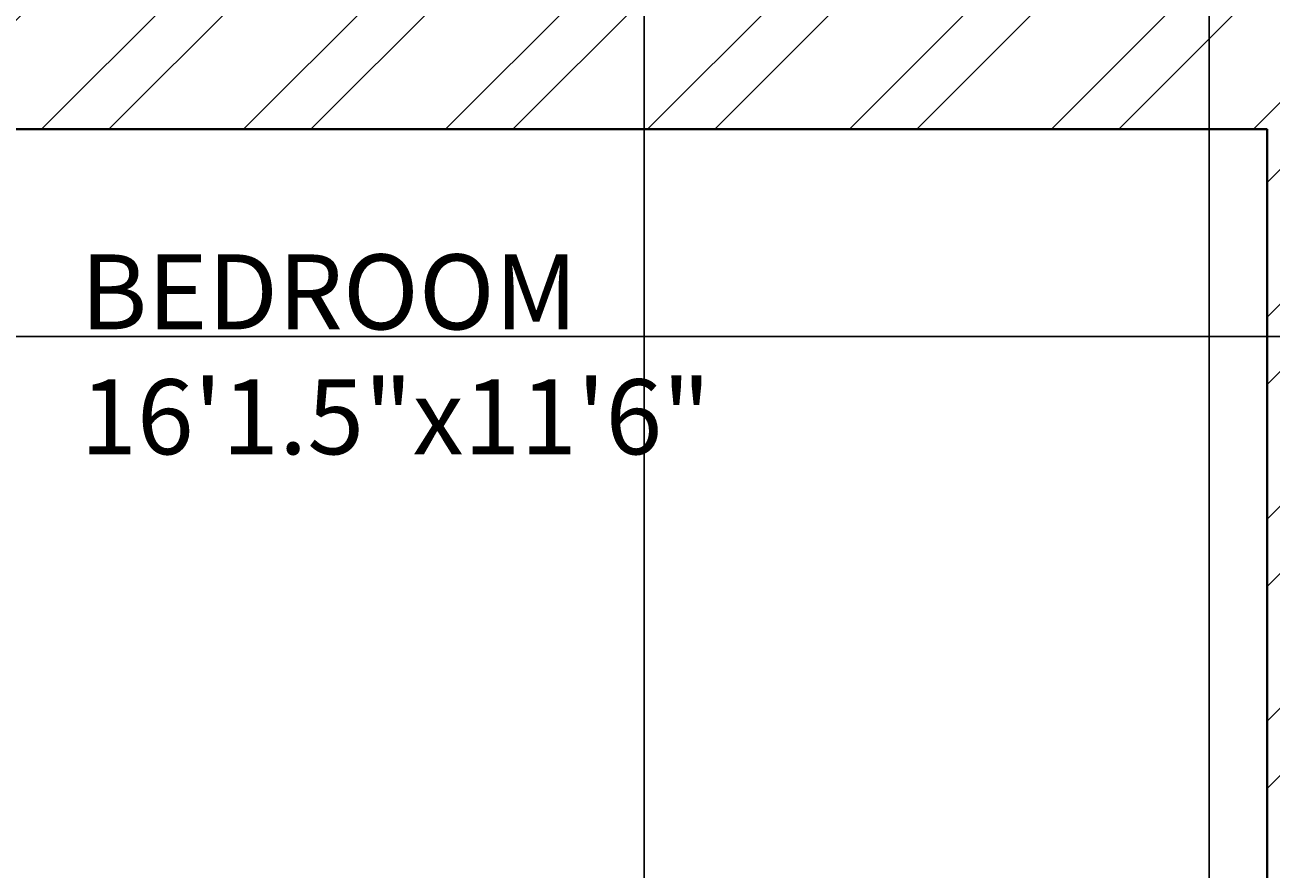
# Model space of a CAD drawing. Units: inches. Extents: x 1601 to 2297, y 1496 to 2631.
# Tile 13 of 57: x 1806 to 1889, y 1973 to 2029. Entities that reach past the tile are written whole.
import ezdxf

# ---------------------------------------------------------------- set-up
doc = ezdxf.new("R2010")
doc.units = ezdxf.units.IN
for name, color, linetype, lineweight in [('A-ANNO-DIMS', 2, 'Continuous', 18), ('A-AREA-IDEN', 7, 'Continuous', 18), ('A-WALL', 7, 'Continuous', 40), ('A-WALL-PATT', 215, 'Continuous', 13)]:
    doc.layers.add(name, color=color, linetype=linetype, lineweight=lineweight)
doc.styles.get("Standard").update_dxf_attribs({"font": 'arial.ttf'})
doc.dimstyles.get("Standard").update_dxf_attribs({"dimtxt": 0.18, "dimasz": 0.18, "dimexe": 0.18, "dimexo": 0.0625, "dimgap": 0.09, "dimtad": 0, "dimtih": 1, "dimtoh": 1, "dimdec": 4, "dimzin": 0, "dimdsep": 46, "dimtxsty": 'Standard', "dimcen": 0.09, "dimadec": 0, "dimazin": 0, "dimtfac": 1, "dimtdec": 4, "dimtofl": 0, "dimtmove": 0, "dimatfit": 3, "dimfxl": 1, "dimtolj": 1, "dimtzin": 0, "dimarcsym": 0})

# ---------------------------------------------------------------- blocks, each defined once
blk = doc.blocks.new('*D45')
at = {"layer": 'A-ANNO-DIMS', "color": 0, "lineweight": -2, "transparency": 16777216}
for p, q in [((1958.975, 2040.303), (1637.307, 2040.303)), ((1637.487, 2040.123), (1637.487, 2024.571)), ((1637.487, 2008.656), (1637.487, 2024.207)), ((1958.975, 2008.476), (1637.307, 2008.476))]:
    blk.add_line(p, q, dxfattribs=at)
at = {"layer": 'A-ANNO-DIMS', "color": 0, "transparency": 16777216}
for points in [[(1637.457, 2040.123), (1637.517, 2040.123), (1637.487, 2040.303)], [(1637.457, 2008.656), (1637.517, 2008.656), (1637.487, 2008.476)]]:
    blk.add_solid(points, dxfattribs=at)
at = {"layer": 'Defpoints', "color": 0, "transparency": 16777216}
for p in [(1637.487, 2040.303), (1959.037, 2040.303), (1959.037, 2008.476)]:
    blk.add_point(p, dxfattribs=at)
at = {"layer": 'A-ANNO-DIMS', "color": 0, "transparency": 16777216, "insert": (1637.487, 2024.389), "char_height": 0.18, "attachment_point": 5}
blk.add_mtext('\\A1;31.83', dxfattribs=at)
blk = doc.blocks.new('*D46')
at = {"layer": 'A-ANNO-DIMS', "color": 0, "lineweight": -2, "transparency": 16777216}
for p, q in [((1846.995, 2347.763), (1846.995, 1513.748)), ((1884.677, 2347.763), (1884.677, 1513.748)), ((1847.175, 1513.928), (1865.442, 1513.928)), ((1884.497, 1513.928), (1866.23, 1513.928))]:
    blk.add_line(p, q, dxfattribs=at)
at = {"layer": 'A-ANNO-DIMS', "color": 0, "transparency": 16777216}
for points in [[(1847.175, 1513.958), (1847.175, 1513.898), (1846.995, 1513.928)], [(1884.497, 1513.958), (1884.497, 1513.898), (1884.677, 1513.928)]]:
    blk.add_solid(points, dxfattribs=at)
at = {"layer": 'Defpoints', "color": 0, "transparency": 16777216}
for p in [(1846.995, 2347.825), (1884.677, 2347.825), (1884.677, 1513.928)]:
    blk.add_point(p, dxfattribs=at)
at = {"layer": 'A-ANNO-DIMS', "color": 0, "transparency": 16777216, "insert": (1865.836, 1513.928), "char_height": 0.18, "attachment_point": 5}
blk.add_mtext('\\A1;37.68', dxfattribs=at)

msp = doc.modelspace()

# ---------------------------------------------------------------- hatches: boundary and pattern name
at = {"layer": 'A-WALL-PATT'}
h = msp.add_hatch(dxfattribs=at)
h.set_pattern_fill('ANSI32', color=256)
h.paths.add_polyline_path([(1842.0336, 2528.0767), (1842.0336, 2532.3254), (1686.0373, 2532.3254), (1686.0373, 2492.9493), (1695.0373, 2492.9493), (1695.0373, 2523.3254), (1827.0373, 2523.3254), (1827.0373, 2416.8254), (1834.6225, 2416.8254), (1834.6225, 2419.0754), (1834.6225, 2421.3254), (1831.5373, 2421.3254), (1831.5373, 2523.3254), (1842.0336, 2523.3254)])
h.paths.add_polyline_path([(1695.0373, 2432.9493), (1686.0373, 2432.9493), (1686.0373, 2325.989), (1695.0373, 2325.989), (1695.0373, 2347.8254), (1827.0373, 2347.8254), (1827.0373, 2287.8254), (1823.2991, 2287.8254), (1823.2991, 2283.3254), (1847.9422, 2283.3254), (1847.9422, 2285.5754), (1847.9422, 2287.8254), (1831.5373, 2287.8254), (1831.5373, 2347.8254), (1846.9946, 2347.8254), (1846.9946, 2350.0754), (1846.9946, 2352.3254), (1695.0373, 2352.3254)])
h.paths.add_polyline_path([(1807.1169, 1573.5395), (2055.0405, 1573.5395), (2055.0405, 1610.6322), (1807.1169, 1610.6322)], flags=9)
h.paths.add_polyline_path([(1841.1631, 1712.7967), (1870.3957, 1712.7967), (1870.3957, 1731.454), (1841.1631, 1731.454)], flags=9)
h.paths.add_polyline_path([(2144.3862, 1772.185), (2191.0233, 1772.185), (2191.0233, 1790.8423), (2144.3862, 1790.8423)], flags=9)
h.paths.add_polyline_path([(2143.0128, 1827.3312), (2177.9958, 1827.3312), (2177.9958, 1845.9886), (2143.0128, 1845.9886)], flags=9)
h.paths.add_polyline_path([(2041.2439, 1833.5691), (2070.8516, 1833.5691), (2070.8516, 1852.2264), (2041.2439, 1852.2264)], flags=9)
h.paths.add_polyline_path([(2097.2791, 1947.0598), (2134.2061, 1947.0598), (2134.2061, 1965.7171), (2097.2791, 1965.7171)], flags=9)
h.paths.add_polyline_path([(2214.995, 1904.3124), (2214.995, 1942.2899), (2196.3376, 1942.2899), (2196.3376, 1904.3124)], flags=9)
h.paths.add_polyline_path([(2186.6284, 2043.8031), (2219.7935, 2043.8031), (2219.7935, 2062.4605), (2186.6284, 2062.4605)], flags=9)
h.paths.add_polyline_path([(2064.0877, 2031.616), (2097.4949, 2031.616), (2097.4949, 2050.2734), (2064.0877, 2050.2734)], flags=9)
h.paths.add_polyline_path([(1973.1349, 1986.0688), (2008.4009, 1986.0688), (2008.4009, 2004.7261), (1973.1349, 2004.7261)], flags=9)
h.paths.add_polyline_path([(1976.3676, 2106.9635), (2005.7469, 2106.9635), (2005.7469, 2125.6209), (1976.3676, 2125.6209)], flags=9)
h.paths.add_polyline_path([(1991.7852, 2180.4863), (2027.0513, 2180.4863), (2027.0513, 2199.1437), (1991.7852, 2199.1437)], flags=9)
h.paths.add_polyline_path([(2106.1801, 2187.9359), (2152.2101, 2187.9359), (2152.2101, 2206.5932), (2106.1801, 2206.5932)], flags=9)
h.paths.add_polyline_path([(2148.6686, 2262.2542), (2182.318, 2262.2542), (2182.318, 2280.9115), (2148.6686, 2280.9115)], flags=9)
h.paths.add_polyline_path([(2041.6327, 2252.8147), (2071.2405, 2252.8147), (2071.2405, 2271.4721), (2041.6327, 2271.4721)], flags=9)
h.paths.add_polyline_path([(2063.9734, 2375.4265), (2100.9004, 2375.4265), (2100.9004, 2394.0839), (2063.9734, 2394.0839)], flags=9)
h.paths.add_polyline_path([(2216.4955, 2330.9748), (2216.4955, 2370.2654), (2197.8381, 2370.2654), (2197.8381, 2330.9748)], flags=9)
h.paths.add_polyline_path([(2179.1416, 2485.8687), (2212.3067, 2485.8687), (2212.3067, 2504.5261), (2179.1416, 2504.5261)], flags=9)
h.paths.add_polyline_path([(2078.7442, 2471.1516), (2112.1514, 2471.1516), (2112.1514, 2489.809), (2078.7442, 2489.809)], flags=9)
h.paths.add_polyline_path([(1915.9631, 2329.4668), (1952.8902, 2329.4668), (1952.8902, 2348.1241), (1915.9631, 2348.1241)], flags=9)
h.paths.add_polyline_path([(1904.3189, 2499.6709), (1940.4512, 2499.6709), (1940.4512, 2518.3282), (1904.3189, 2518.3282)], flags=9)
h.paths.add_polyline_path([(1892.3665, 2100.4595), (1925.6374, 2100.4595), (1925.6374, 2119.1169), (1892.3665, 2119.1169)], flags=9)
h.paths.add_polyline_path([(1909.2984, 1805.9631), (1946.2254, 1805.9631), (1946.2254, 1824.6205), (1909.2984, 1824.6205)], flags=9)
h.paths.add_polyline_path([(1934.6056, 1658.616), (1970.738, 1658.616), (1970.738, 1677.2733), (1934.6056, 1677.2733)], flags=9)
h.paths.add_polyline_path([(1711.2052, 1789.8902), (1750.0456, 1789.8902), (1750.0456, 1808.5476), (1711.2052, 1808.5476)], flags=9)
h.paths.add_polyline_path([(1742.7874, 1854.6743), (1771.9449, 1854.6743), (1771.9449, 1873.3317), (1742.7874, 1873.3317)], flags=9)
h.paths.add_polyline_path([(1807.3592, 1997.7912), (1850.1116, 1997.7912), (1850.1116, 2016.4486), (1807.3592, 2016.4486)], flags=9)
h.paths.add_polyline_path([(1717.4579, 2237.7844), (1760.2103, 2237.7844), (1760.2103, 2256.4417), (1717.4579, 2256.4417)], flags=9)
h.paths.add_polyline_path([(1780.9285, 2324.0623), (1810.086, 2324.0623), (1810.086, 2342.7197), (1780.9285, 2342.7197)], flags=25)
h.paths.add_polyline_path([(1837.696, 2449.2024), (1866.9286, 2449.2024), (1866.9286, 2467.8598), (1837.696, 2467.8598)], flags=9)
h.paths.add_polyline_path([(1712.7752, 2484.9404), (1751.6156, 2484.9404), (1751.6156, 2503.5977), (1712.7752, 2503.5977)], flags=25)
h = msp.add_hatch(dxfattribs=at)
h.set_pattern_fill('ANSI32', color=256)
h.paths.add_polyline_path([(1973.9371, 2211.3254), (1893.0373, 2211.3254), (1893.0373, 2287.8254), (1884.6167, 2287.8254), (1884.6167, 2285.5754), (1884.6167, 2283.3254), (1888.5373, 2283.3254), (1888.5373, 2145.3254), (1695.0373, 2145.3254), (1695.0373, 2173.8724), (1690.5373, 2173.8724), (1686.0373, 2173.8724), (1686.0373, 2136.3254), (1722.5687, 2136.3254), (1722.5687, 2117.4352), (1731.5687, 2117.4352), (1731.5687, 2136.3254), (1893.0373, 2136.3254), (1893.0373, 2202.3254), (1959.0373, 2202.3254), (1959.0373, 2182.1303), (1968.0373, 2182.1303), (1968.0373, 2202.3254), (1973.9371, 2202.3254)])
h.paths.add_polyline_path([(2094.0373, 2274.6364), (2096.4294, 2274.6364), (2096.4294, 2276.8864), (2096.4294, 2279.1364), (2094.0373, 2279.1364), (2094.0373, 2290.8254), (2094.0373, 2295.3254), (2089.5373, 2295.3254), (2089.5373, 2230.8254), (2035.5373, 2230.8254), (2035.5373, 2299.8254), (2031.0373, 2299.8254), (2031.0373, 2211.3254), (2023.0065, 2211.3254), (2023.0065, 2202.3254), (2031.0373, 2202.3254), (2031.0373, 2140.8254), (1968.0373, 2140.8254), (1968.0373, 2145.9106), (1963.5373, 2145.9106), (1959.0373, 2145.9106), (1959.0373, 2116.839), (1963.5373, 2116.839), (1968.0373, 2116.839), (1968.0373, 2131.8254), (2031.0373, 2131.8254), (2031.0373, 2094.3254), (2031.0373, 2085.3254), (2031.0373, 2056.8254), (1968.0373, 2056.8254), (1968.0373, 2070.4947), (1963.5373, 2070.4947), (1959.0373, 2070.4947), (1959.0373, 2040.3029), (1968.0373, 2040.3029), (1968.0373, 2047.8254), (2031.0373, 2047.8254), (2031.0373, 1983.3254), (2031.0373, 1978.8254), (2021.1979, 1978.8254), (2021.1979, 1974.3254), (2031.0373, 1974.3254), (2031.0373, 1954.3528), (2035.5373, 1954.3528), (2035.5373, 1974.3254), (2035.5373, 1981.8254), (2055.5513, 1981.8254), (2055.5513, 1986.3254), (2035.5373, 1986.3254), (2035.5373, 2047.8254), (2040.0373, 2047.8254), (2040.0373, 2085.3254), (2040.0373, 2094.3254), (2040.0373, 2140.8254), (2035.5373, 2140.8254), (2035.5373, 2226.3254), (2089.5373, 2226.3254), (2094.0373, 2226.3254)])
h.paths.add_polyline_path([(2226.0373, 2230.8254), (2134.5373, 2230.8254), (2134.5373, 2233.5437), (2130.0373, 2233.5437), (2130.0373, 2226.3254), (2134.5373, 2226.3254), (2226.0373, 2226.3254)])
h.paths.add_polyline_path([(1807.1169, 1573.5395), (2055.0405, 1573.5395), (2055.0405, 1610.6322), (1807.1169, 1610.6322)], flags=9)
h.paths.add_polyline_path([(1841.1631, 1712.7967), (1870.3957, 1712.7967), (1870.3957, 1731.454), (1841.1631, 1731.454)], flags=9)
h.paths.add_polyline_path([(2144.3862, 1772.185), (2191.0233, 1772.185), (2191.0233, 1790.8423), (2144.3862, 1790.8423)], flags=9)
h.paths.add_polyline_path([(2143.0128, 1827.3312), (2177.9958, 1827.3312), (2177.9958, 1845.9886), (2143.0128, 1845.9886)], flags=9)
h.paths.add_polyline_path([(2041.2439, 1833.5691), (2070.8516, 1833.5691), (2070.8516, 1852.2264), (2041.2439, 1852.2264)], flags=9)
h.paths.add_polyline_path([(2097.2791, 1947.0598), (2134.2061, 1947.0598), (2134.2061, 1965.7171), (2097.2791, 1965.7171)], flags=9)
h.paths.add_polyline_path([(2214.995, 1904.3124), (2214.995, 1942.2899), (2196.3376, 1942.2899), (2196.3376, 1904.3124)], flags=9)
h.paths.add_polyline_path([(2186.6284, 2043.8031), (2219.7935, 2043.8031), (2219.7935, 2062.4605), (2186.6284, 2062.4605)], flags=9)
h.paths.add_polyline_path([(2064.0877, 2031.616), (2097.4949, 2031.616), (2097.4949, 2050.2734), (2064.0877, 2050.2734)], flags=9)
h.paths.add_polyline_path([(1973.1349, 1986.0688), (2008.4009, 1986.0688), (2008.4009, 2004.7261), (1973.1349, 2004.7261)], flags=25)
h.paths.add_polyline_path([(1976.3676, 2106.9635), (2005.7469, 2106.9635), (2005.7469, 2125.6209), (1976.3676, 2125.6209)], flags=25)
h.paths.add_polyline_path([(1991.7852, 2180.4863), (2027.0513, 2180.4863), (2027.0513, 2199.1437), (1991.7852, 2199.1437)], flags=25)
h.paths.add_polyline_path([(2106.1801, 2187.9359), (2152.2101, 2187.9359), (2152.2101, 2206.5932), (2106.1801, 2206.5932)], flags=9)
h.paths.add_polyline_path([(2148.6686, 2262.2542), (2182.318, 2262.2542), (2182.318, 2280.9115), (2148.6686, 2280.9115)], flags=9)
h.paths.add_polyline_path([(2041.6327, 2252.8147), (2071.2405, 2252.8147), (2071.2405, 2271.4721), (2041.6327, 2271.4721)], flags=25)
h.paths.add_polyline_path([(2063.9734, 2375.4265), (2100.9004, 2375.4265), (2100.9004, 2394.0839), (2063.9734, 2394.0839)], flags=9)
h.paths.add_polyline_path([(2216.4955, 2330.9748), (2216.4955, 2370.2654), (2197.8381, 2370.2654), (2197.8381, 2330.9748)], flags=9)
h.paths.add_polyline_path([(2179.1416, 2485.8687), (2212.3067, 2485.8687), (2212.3067, 2504.5261), (2179.1416, 2504.5261)], flags=9)
h.paths.add_polyline_path([(2078.7442, 2471.1516), (2112.1514, 2471.1516), (2112.1514, 2489.809), (2078.7442, 2489.809)], flags=9)
h.paths.add_polyline_path([(1915.9631, 2329.4668), (1952.8902, 2329.4668), (1952.8902, 2348.1241), (1915.9631, 2348.1241)], flags=9)
h.paths.add_polyline_path([(1904.3189, 2499.6709), (1940.4512, 2499.6709), (1940.4512, 2518.3282), (1904.3189, 2518.3282)], flags=9)
h.paths.add_polyline_path([(1892.3665, 2100.4595), (1925.6374, 2100.4595), (1925.6374, 2119.1169), (1892.3665, 2119.1169)], flags=9)
h.paths.add_polyline_path([(1909.2984, 1805.9631), (1946.2254, 1805.9631), (1946.2254, 1824.6205), (1909.2984, 1824.6205)], flags=9)
h.paths.add_polyline_path([(1934.6056, 1658.616), (1970.738, 1658.616), (1970.738, 1677.2733), (1934.6056, 1677.2733)], flags=9)
h.paths.add_polyline_path([(1711.2052, 1789.8902), (1750.0456, 1789.8902), (1750.0456, 1808.5476), (1711.2052, 1808.5476)], flags=9)
h.paths.add_polyline_path([(1742.7874, 1854.6743), (1771.9449, 1854.6743), (1771.9449, 1873.3317), (1742.7874, 1873.3317)], flags=9)
h.paths.add_polyline_path([(1807.3592, 1997.7912), (1850.1116, 1997.7912), (1850.1116, 2016.4486), (1807.3592, 2016.4486)], flags=9)
h.paths.add_polyline_path([(1717.4579, 2237.7844), (1760.2103, 2237.7844), (1760.2103, 2256.4417), (1717.4579, 2256.4417)], flags=25)
h.paths.add_polyline_path([(1780.9285, 2324.0623), (1810.086, 2324.0623), (1810.086, 2342.7197), (1780.9285, 2342.7197)], flags=9)
h.paths.add_polyline_path([(1837.696, 2449.2024), (1866.9286, 2449.2024), (1866.9286, 2467.8598), (1837.696, 2467.8598)], flags=9)
h.paths.add_polyline_path([(1712.7752, 2484.9404), (1751.6156, 2484.9404), (1751.6156, 2503.5977), (1712.7752, 2503.5977)], flags=9)
h = msp.add_hatch(dxfattribs=at)
h.set_pattern_fill('ANSI32', color=256)
h.paths.add_polyline_path([(2230.5373, 1861.8254), (2182.5373, 1861.8254), (2182.5373, 1885.3637), (2178.0373, 1885.3637), (2178.0373, 1861.8254), (2166.0373, 1861.8254), (2134.5373, 1861.8254), (2130.0373, 1861.8254), (2130.0373, 1841.4682), (2126.8833, 1841.4682), (2126.8833, 1836.9682), (2130.0373, 1836.9682), (2130.0373, 1822.7302), (2134.5373, 1822.7302), (2134.5373, 1857.3254), (2166.0373, 1857.3254), (2226.0373, 1857.3254), (2226.0373, 1846.1155), (2230.5373, 1846.1155)])
h.paths.add_polyline_path([(2226.0373, 1797.3254), (2134.5373, 1797.3254), (2134.5373, 1800.6636), (2132.2873, 1800.6636), (2130.0373, 1800.6636), (2130.0373, 1797.3254), (2130.0373, 1792.8254), (2167.7264, 1792.8254), (2226.0373, 1792.8254)])
h.paths.add_polyline_path([(2230.5373, 1822.1155), (2226.0373, 1822.1155), (2226.0373, 1760.8563), (2230.5373, 1760.8563)])
h.paths.add_polyline_path([(2230.5373, 1700.8563), (2226.0373, 1700.8563), (2226.0373, 1644.3254), (2140.2517, 1644.3254), (2140.2517, 1635.3254), (2230.5373, 1635.3254)])
h.paths.add_polyline_path([(2080.2517, 1639.8254), (2080.2517, 1644.3254), (2035.5373, 1644.3254), (2035.5373, 1792.8254), (2094.0373, 1792.8254), (2094.0373, 1797.3254), (2094.0373, 1836.9682), (2097.1057, 1836.9682), (2097.1057, 1839.2182), (2097.1057, 1841.4682), (2094.0373, 1841.4682), (2094.0373, 1862.2276), (2089.5373, 1862.2276), (2089.5373, 1797.3254), (2035.5373, 1797.3254), (2035.5373, 1857.3254), (2035.5373, 1885.0916), (2031.0373, 1885.0916), (2031.0373, 1710.3254), (2012.329, 1710.3254), (2012.329, 1701.3254), (2031.0373, 1701.3254), (2031.0373, 1644.3254), (2031.0373, 1635.3254), (2080.2517, 1635.3254)])
h.paths.add_polyline_path([(1836.0373, 1653.2033), (1842.6171, 1653.2033), (1842.6171, 1657.7033), (1842.6171, 1662.2033), (1831.5373, 1662.2033), (1831.5373, 1764.2033), (1835.3881, 1764.2033), (1835.3881, 1766.4533), (1835.3881, 1768.7033), (1831.5373, 1768.7033), (1827.0373, 1768.7033), (1827.0373, 1662.2033), (1827.0373, 1635.3254), (1836.0373, 1635.3254)])
h.paths.add_polyline_path([(1893.0373, 1701.3254), (1907.193, 1701.3254), (1907.193, 1705.8254), (1907.193, 1710.3254), (1893.0373, 1710.3254), (1893.0373, 1819.8254), (1882.6444, 1819.8254), (1882.6444, 1817.5754), (1882.6444, 1815.3254), (1888.5373, 1815.3254), (1888.5373, 1662.2033), (1884.0373, 1662.2033), (1866.6171, 1662.2033), (1866.6171, 1653.2033), (1882.391, 1653.2033), (1884.0373, 1653.2033), (1884.0373, 1635.3254), (1893.0373, 1635.3254)])
h.paths.add_polyline_path([(1739.3335, 1639.8254), (1739.3335, 1644.3254), (1695.0373, 1644.3254), (1695.0373, 1702.0135), (1690.5373, 1702.0135), (1686.0373, 1702.0135), (1686.0373, 1635.3254), (1739.3335, 1635.3254)])
h.paths.add_polyline_path([(1827.0373, 1644.3254), (1799.3335, 1644.3254), (1799.3335, 1635.3254), (1827.0373, 1635.3254)])
h.paths.add_polyline_path([(1695.0373, 1815.3254), (1849.2759, 1815.3254), (1849.2759, 1819.8254), (1807.5373, 1819.8254), (1807.5373, 1879.8254), (1851.1533, 1879.8254), (1851.1533, 1882.0754), (1851.1533, 1884.3254), (1799.3405, 1884.3254), (1799.3405, 1882.0754), (1799.3405, 1879.8254), (1803.0373, 1879.8254), (1803.0373, 1819.8254), (1695.0373, 1819.8254), (1695.0373, 1835.0458), (1690.5373, 1835.0458), (1686.0373, 1835.0458), (1686.0373, 1766.1753), (1695.0373, 1766.1753)])
h.paths.add_polyline_path([(1775.8157, 1884.3254), (1695.0373, 1884.3254), (1695.0373, 1912.9526), (1690.5373, 1912.9526), (1686.0373, 1912.9526), (1686.0373, 1859.0458), (1695.0373, 1859.0458), (1695.0373, 1879.8254), (1775.8157, 1879.8254)])
h.paths.add_polyline_path([(1893.0373, 2031.3254), (1731.5687, 2031.3254), (1731.5687, 2057.4352), (1722.5687, 2057.4352), (1722.5687, 2031.3254), (1686.0373, 2031.3254), (1686.0373, 1972.9526), (1695.0373, 1972.9526), (1695.0373, 2022.3254), (1888.5373, 2022.3254), (1888.5373, 1884.3254), (1883.4996, 1884.3254), (1883.4996, 1879.8254), (1893.0373, 1879.8254), (1893.0373, 1974.3254), (1976.6199, 1974.3254), (1976.6199, 1978.8254), (1968.0373, 1978.8254), (1968.0373, 1983.3254), (1968.0373, 2008.4756), (1963.5373, 2008.4756), (1959.0373, 2008.4756), (1959.0373, 1983.3254), (1893.0373, 1983.3254)])
h.paths.add_polyline_path([(2230.5373, 2140.4745), (2226.0373, 2140.4745), (2226.0373, 2094.3254), (2040.0373, 2094.3254), (2040.0373, 2085.3254), (2178.0373, 2085.3254), (2178.0373, 2065.6965), (2182.5373, 2065.6965), (2182.5373, 2085.3254), (2226.0373, 2085.3254), (2226.0373, 1986.3254), (2211.2679, 1986.3254), (2211.2679, 1981.8254), (2230.5373, 1981.8254)])
h.paths.add_polyline_path([(2187.6292, 1986.3254), (2182.5373, 1986.3254), (2182.5373, 2029.6965), (2178.0373, 2029.6965), (2178.0373, 1986.3254), (2099.05, 1986.3254), (2099.05, 1981.8254), (2178.0373, 1981.8254), (2178.0373, 1969.3637), (2182.5373, 1969.3637), (2182.5373, 1981.8254), (2187.6292, 1981.8254), (2187.6292, 1984.0754)])
h.paths.add_polyline_path([(1807.1169, 1573.5395), (2055.0405, 1573.5395), (2055.0405, 1610.6322), (1807.1169, 1610.6322)], flags=9)
h.paths.add_polyline_path([(1841.1631, 1712.7967), (1870.3957, 1712.7967), (1870.3957, 1731.454), (1841.1631, 1731.454)], flags=9)
h.paths.add_polyline_path([(2144.3862, 1772.185), (2191.0233, 1772.185), (2191.0233, 1790.8423), (2144.3862, 1790.8423)], flags=9)
h.paths.add_polyline_path([(2143.0128, 1827.3312), (2177.9958, 1827.3312), (2177.9958, 1845.9886), (2143.0128, 1845.9886)], flags=25)
h.paths.add_polyline_path([(2041.2439, 1833.5691), (2070.8516, 1833.5691), (2070.8516, 1852.2264), (2041.2439, 1852.2264)], flags=25)
h.paths.add_polyline_path([(2097.2791, 1947.0598), (2134.2061, 1947.0598), (2134.2061, 1965.7171), (2097.2791, 1965.7171)], flags=9)
h.paths.add_polyline_path([(2214.995, 1904.3124), (2214.995, 1942.2899), (2196.3376, 1942.2899), (2196.3376, 1904.3124)], flags=9)
h.paths.add_polyline_path([(2186.6284, 2043.8031), (2219.7935, 2043.8031), (2219.7935, 2062.4605), (2186.6284, 2062.4605)], flags=25)
h.paths.add_polyline_path([(2064.0877, 2031.616), (2097.4949, 2031.616), (2097.4949, 2050.2734), (2064.0877, 2050.2734)], flags=25)
h.paths.add_polyline_path([(1973.1349, 1986.0688), (2008.4009, 1986.0688), (2008.4009, 2004.7261), (1973.1349, 2004.7261)], flags=9)
h.paths.add_polyline_path([(1976.3676, 2106.9635), (2005.7469, 2106.9635), (2005.7469, 2125.6209), (1976.3676, 2125.6209)], flags=9)
h.paths.add_polyline_path([(1991.7852, 2180.4863), (2027.0513, 2180.4863), (2027.0513, 2199.1437), (1991.7852, 2199.1437)], flags=9)
h.paths.add_polyline_path([(2106.1801, 2187.9359), (2152.2101, 2187.9359), (2152.2101, 2206.5932), (2106.1801, 2206.5932)], flags=9)
h.paths.add_polyline_path([(2148.6686, 2262.2542), (2182.318, 2262.2542), (2182.318, 2280.9115), (2148.6686, 2280.9115)], flags=9)
h.paths.add_polyline_path([(2041.6327, 2252.8147), (2071.2405, 2252.8147), (2071.2405, 2271.4721), (2041.6327, 2271.4721)], flags=9)
h.paths.add_polyline_path([(2063.9734, 2375.4265), (2100.9004, 2375.4265), (2100.9004, 2394.0839), (2063.9734, 2394.0839)], flags=9)
h.paths.add_polyline_path([(2216.4955, 2330.9748), (2216.4955, 2370.2654), (2197.8381, 2370.2654), (2197.8381, 2330.9748)], flags=9)
h.paths.add_polyline_path([(2179.1416, 2485.8687), (2212.3067, 2485.8687), (2212.3067, 2504.5261), (2179.1416, 2504.5261)], flags=9)
h.paths.add_polyline_path([(2078.7442, 2471.1516), (2112.1514, 2471.1516), (2112.1514, 2489.809), (2078.7442, 2489.809)], flags=9)
h.paths.add_polyline_path([(1915.9631, 2329.4668), (1952.8902, 2329.4668), (1952.8902, 2348.1241), (1915.9631, 2348.1241)], flags=9)
h.paths.add_polyline_path([(1904.3189, 2499.6709), (1940.4512, 2499.6709), (1940.4512, 2518.3282), (1904.3189, 2518.3282)], flags=9)
h.paths.add_polyline_path([(1892.3665, 2100.4595), (1925.6374, 2100.4595), (1925.6374, 2119.1169), (1892.3665, 2119.1169)], flags=9)
h.paths.add_polyline_path([(1909.2984, 1805.9631), (1946.2254, 1805.9631), (1946.2254, 1824.6205), (1909.2984, 1824.6205)], flags=9)
h.paths.add_polyline_path([(1934.6056, 1658.616), (1970.738, 1658.616), (1970.738, 1677.2733), (1934.6056, 1677.2733)], flags=9)
h.paths.add_polyline_path([(1711.2052, 1789.8902), (1750.0456, 1789.8902), (1750.0456, 1808.5476), (1711.2052, 1808.5476)], flags=25)
h.paths.add_polyline_path([(1742.7874, 1854.6743), (1771.9449, 1854.6743), (1771.9449, 1873.3317), (1742.7874, 1873.3317)], flags=25)
h.paths.add_polyline_path([(1807.3592, 1997.7912), (1850.1116, 1997.7912), (1850.1116, 2016.4486), (1807.3592, 2016.4486)], flags=25)
h.paths.add_polyline_path([(1717.4579, 2237.7844), (1760.2103, 2237.7844), (1760.2103, 2256.4417), (1717.4579, 2256.4417)], flags=9)
h.paths.add_polyline_path([(1780.9285, 2324.0623), (1810.086, 2324.0623), (1810.086, 2342.7197), (1780.9285, 2342.7197)], flags=9)
h.paths.add_polyline_path([(1837.696, 2449.2024), (1866.9286, 2449.2024), (1866.9286, 2467.8598), (1837.696, 2467.8598)], flags=9)
h.paths.add_polyline_path([(1712.7752, 2484.9404), (1751.6156, 2484.9404), (1751.6156, 2503.5977), (1712.7752, 2503.5977)], flags=9)

# ---------------------------------------------------------------- linework, layer by layer
at = {"layer": 'A-WALL'}
for p, q in [((1695.0373, 2022.3254), (1888.5373, 2022.3254)), ((1888.5373, 2022.3254), (1888.5373, 1884.3254))]:
    msp.add_line(p, q, dxfattribs=at)

# ---------------------------------------------------------------- texts
at = {"layer": 'A-AREA-IDEN', "insert": (1809.3697, 2013.9639), "char_height": 5, "attachment_point": 1}
msp.add_mtext_dynamic_manual_height_columns('BEDROOM\\P16\'1.5"x11\'6"', width=143.923966, gutter_width=12.5, heights=[0], dxfattribs=at)

# ---------------------------------------------------------------- dimensions: what is measured, and where the dimension line sits
at = {"layer": 'A-ANNO-DIMS'}
dim = msp.add_linear_dim(base=(1884.6773, 1513.9279), p1=(1846.9946, 2347.8254), p2=(1884.6773, 2347.8254), dimstyle='Standard', override={"dimdec": 2, "dimlfac": 1, "dimrnd": 0, "dimzin": 0, "dimdsep": 46, "dimlunit": 2}, dxfattribs=at)
dim.commit()
dim.dimension.update_dxf_attribs({"geometry": '*D46', "text_midpoint": (1865.836, 1513.9279)})
dim = msp.add_linear_dim(base=(1637.4873, 2040.3029), p1=(1959.0373, 2008.4756), p2=(1959.0373, 2040.3029), angle=90, dimstyle='Standard', override={"dimdec": 2, "dimlfac": 1, "dimrnd": 0, "dimzin": 0, "dimdsep": 46, "dimlunit": 2}, dxfattribs=at)
dim.commit()
dim.dimension.update_dxf_attribs({"geometry": '*D45', "text_midpoint": (1637.4873, 2024.3893)})

doc.saveas('drawing.dxf')
